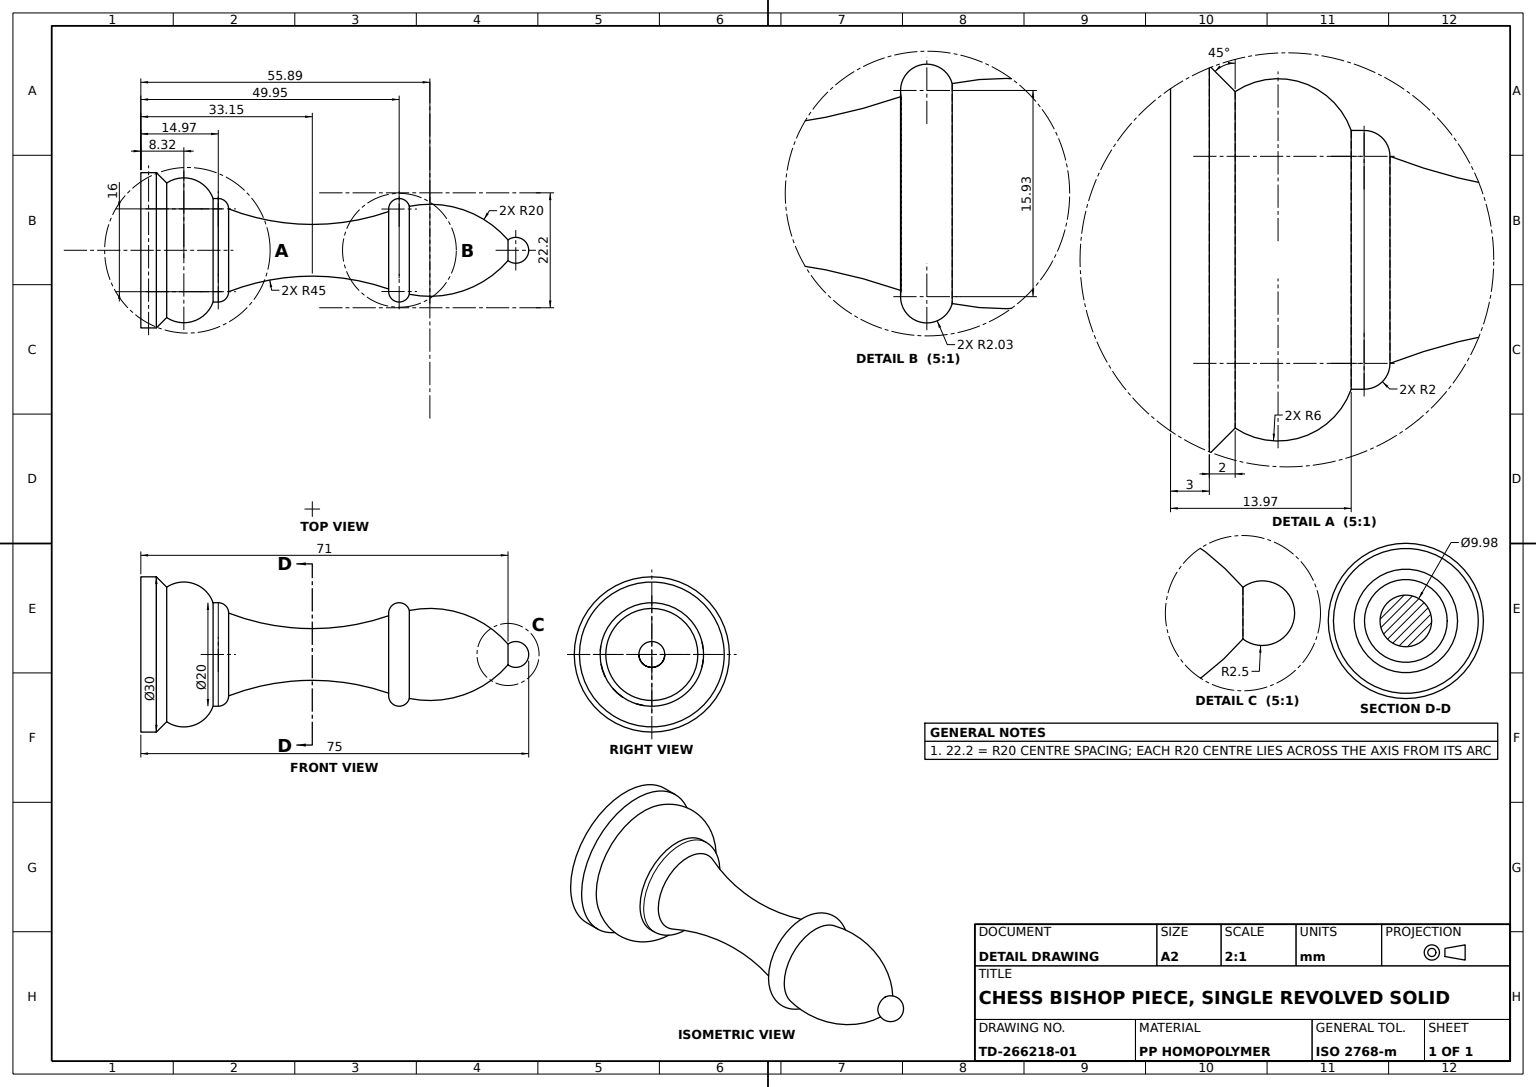
from build123d import *


with BuildPart() as part:
    # Bishop Profile Sketch → Bishop Body Revolve (revolve)
    with BuildSketch(Plane.XY, mode=Mode.PRIVATE) as bishop_body_revolve_sk:
        with BuildLine():
            Line((0, 0), (0, 75))
            ThreePointArc((0, 75), (2.236067977, 73.618033989), (2, 71))
            ThreePointArc((2, 71), (7.831216806, 62.335784437), (8.5, 51.91347904))
            ThreePointArc((8.5, 51.91347904), (9.937529812, 49.451720204), (7.5, 47.97347904))
            ThreePointArc((7.5, 47.97347904), (4.995920105, 32.429058396), (8, 16.97347904))
            ThreePointArc((8, 16.97347904), (9.414213562, 16.387692602), (10, 14.97347904))
            Line((10, 14.97347904), (10, 13.97347904))
            ThreePointArc((10, 13.97347904), (13.69041576, 10.219036018), (13, 5))
            Line((13, 5), (15, 3))
            Line((15, 3), (15, 0))
            Line((15, 0), (0, 0))
        make_face()
    revolve(bishop_body_revolve_sk.sketch.rotate(Axis((0, 0, 0), (0, 1, 0)), 90), axis=Axis((0, 0, 0), (0, 1, 0)))


solid = part.part
